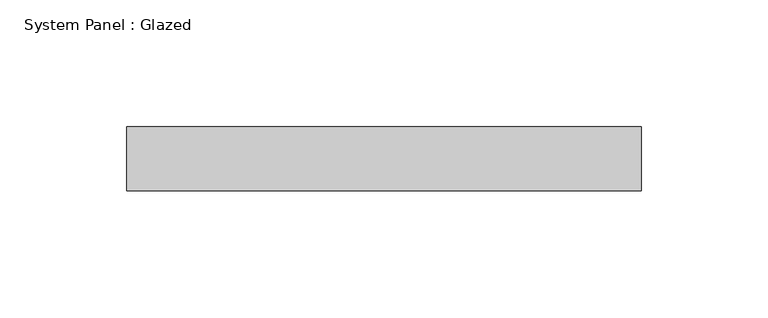
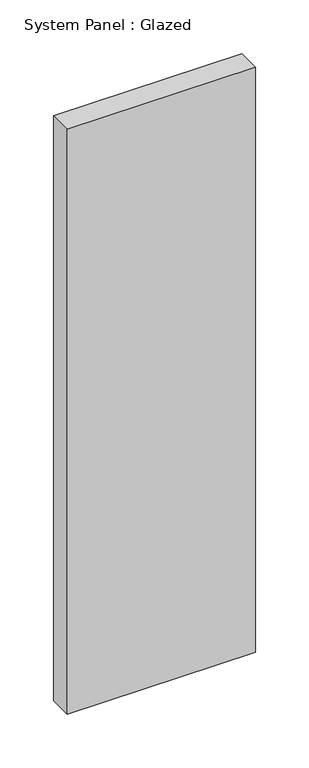
"""IFC4 building model written with IfcOpenShell, lengths in millimetres: plate geometry, System Panel : Glazed."""

from ifc_helpers import new_model, si_unit, origin, origin_with_axes, place, context, project, spatial, polyline, outline, extrude, source, transform, mapped, element, save


def system_panel_glazed_d46f60ed(model_context):
    return source(origin(), model_context, "Body", "SweptSolid", [
        extrude(outline(polyline([(101.6, 19.05), (-101.6, 19.05), (-101.6, 44.45), (101.6, 44.45), (101.6, 19.05)])), origin_with_axes(), (0.0, 0.0, 1.0), 666.75),
    ])


if __name__ == "__main__":
    model = new_model("IFC4")
    model_context = context("Model", 3, world=origin())
    ifc_project = project(units=[si_unit("LENGTHUNIT", "METRE", prefix="MILLI")], contexts=[model_context])
    site = spatial("IfcSite", under=ifc_project)
    building = spatial("IfcBuilding", under=site)
    placement = place(None, origin())
    system_panel_glazed_shape = system_panel_glazed_d46f60ed(model_context)
    element("IfcPlate", 1, ObjectType="System Panel : Glazed", at=placement, inside=building, context=model_context, shape_type="MappedRepresentation", body=[
        mapped(system_panel_glazed_shape, transform((0.0, 0.0, 0.0), x_axis=(1.0, 0.0, 0.0), y_axis=(0.0, 1.0, 0.0), z_axis=(0.0, 0.0, 1.0))),
    ])
    save(model, "model.ifc")

# Revit data of these elements
# Type "System Panel : Glazed"
#   Construction Type Id = "GSP4R"
#   Analytic Construction = "1/8 in Pilkington single glazing"
#   Visual Light Transmittance = 0.9
#   Solar Heat Gain Coefficient = 0.86
#   Heat Transfer Coefficient (U) = 1.18115 BTU/(h·ft²·°F)
#   Define Thermal Properties by = 1
# Element 1 (IfcPlate, "System Panel : Glazed")
#   Materials on its faces: "Glass"
# Materials
#   "Glass": class "Glass", colour RGB 0 128 192, transparency 0.75, Description = "Soda Lime Glass", Cost = 0
